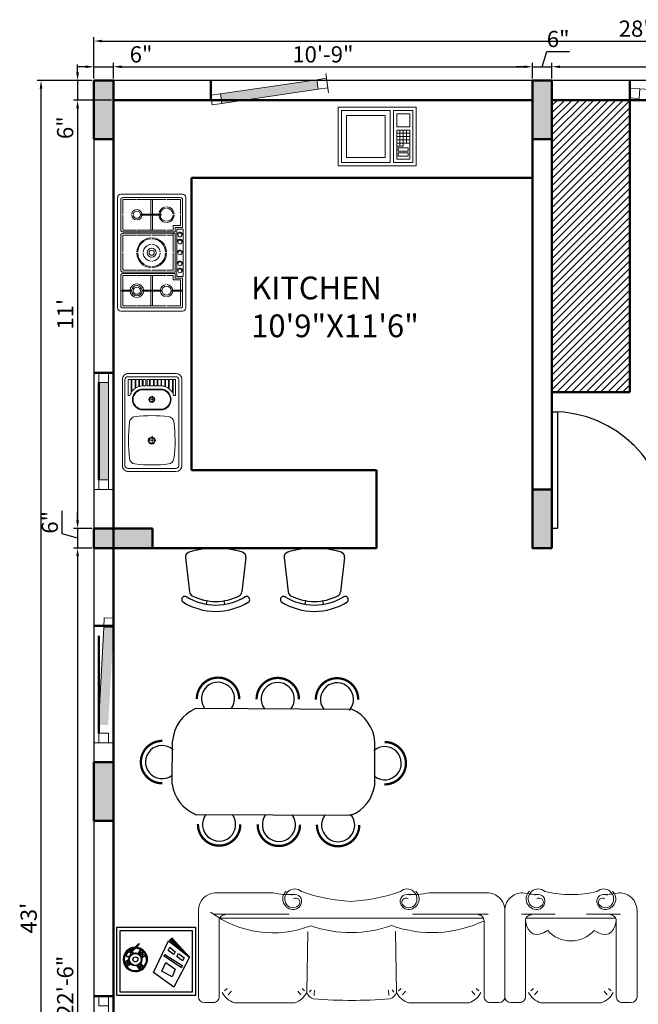
# Model space of a CAD drawing. Units: inches. Extents: x 3064 to 19385, y 846 to 15425.
# Tile 28 of 108: x 4742 to 4932, y 1108 to 1411. Entities that reach past the tile are written whole.
import ezdxf

# ---------------------------------------------------------------- set-up
doc = ezdxf.new("R2010")
doc.units = ezdxf.units.IN
for name, color, linetype, lineweight in [('A-ANNO-DIMS', 2, 'Continuous', 18), ('A-AREA-IDEN', 3, 'Continuous', 18), ('A-COLS', 1, 'Continuous', 35), ('A-DOOR', 3, 'Continuous', 25), ('A-EQPM', 8, 'Continuous', 18), ('A-FLOR-FIXT', 9, 'Continuous', 18), ('A-FURN', 8, 'Continuous', 18), ('A-FURN-PATT', 252, 'Continuous', 13), ('A-GLAZ', 4, 'Continuous', 18), ('A-WALL', 7, 'Continuous', 50), ('C-PROP', 6, 'Continuous', 25)]:
    doc.layers.add(name, color=color, linetype=linetype, lineweight=lineweight)
for name, color, linetype in [('BLO', 135, 'Continuous'), ('FUR', 42, 'Continuous'), ('NOITHAT', 21, 'Continuous'), ('Win', 152, 'Continuous')]:
    doc.layers.add(name, color=color, linetype=linetype)
doc.styles.get("Standard").update_dxf_attribs({"font": 'arial.ttf'})
doc.dimstyles.new('ISO-25', dxfattribs={"dimtxt": 9, "dimasz": 2.5, "dimexe": 1.25, "dimexo": 0.625, "dimtad": 1, "dimdec": 1, "dimlunit": 3, "dimtxsty": 'Standard', "dimcen": 2.5, "dimadec": 0, "dimazin": 0, "dimtfac": 1, "dimtdec": 1, "dimtmove": 0, "dimatfit": 3, "dimfxl": 1, "dimarcsym": 0})

# ---------------------------------------------------------------- blocks, each defined once
blk = doc.blocks.new('*U3')
for p, q in [((0, 0), (0, -6)), ((36, 0), (36, -6))]:
    blk.add_line(p, q)
blk.add_lwpolyline([(0, 0), (0, 36), (1.75, 36), (1.75, 0)], close=True)
blk.add_arc((0, 0), 36, 0, 90)
blk = doc.blocks.new('din')
at = {"layer": 'FUR', "ltscale": 0.25}
for p, q in [((70.23, 15.24), (9.28, 15.24)), ((0, 3.44), (0, -13.56)), ((79.14, 3.44), (79.14, -13.56)), ((8.91, -26.16), (70.23, -26.16))]:
    blk.add_line(p, q, dxfattribs=at)
at = {"layer": 'FUR', "ltscale": 0.25, "const_width": 0.9}
for points in [[(22.5, 19.02, 1.012537), (5.94, 19.02, 1.012537)], [(45.67, 19.02, 1.012537), (29.11, 19.02, 1.012537)], [(69.02, 19.02, 1.012537), (52.46, 19.02, 1.012537)], [(-3.79, 3.1, 1.012537), (-3.79, -13.47, 1.012537)], [(83.08, 3.1, -1.012537), (83.08, -13.47, -1.012537)], [(23.18, -29.95, -1.012537), (6.61, -29.95, -1.012537)], [(46.34, -29.95, -1.012537), (29.78, -29.95, -1.012537)], [(69.7, -29.95, -1.012537), (53.14, -29.95, -1.012537)]]:
    blk.add_lwpolyline(points, format="xyb", dxfattribs=at)
at = {"layer": 'FUR', "ltscale": 0.25}
for centre, radius, start, end in [((14.22, 19.13), 6.48, 323.1301, 221.2163), ((37.39, 19.13), 6.48, 323.1301, 216.8699), ((60.74, 19.13), 6.48, 323.1301, 216.8699), ((14.55, 1.54), 14.67, 111.0491, 172.5731), ((64.59, 1.54), 14.67, 7.4269, 68.9509), ((-3.89, -5.18), 6.48, 53.1301, 311.2163), ((83.18, -5.18), 6.48, 228.7837, 126.8699), ((15.28, -12.21), 15.34, 185.0602, 245.4675), ((63.86, -12.21), 15.34, 294.5325, 354.9398), ((14.89, -30.05), 6.48, 138.7837, 36.8699), ((38.06, -30.05), 6.48, 143.1301, 36.8699), ((61.42, -30.05), 6.48, 143.1301, 36.8699)]:
    blk.add_arc(centre, radius, start, end, dxfattribs=at)
blk = doc.blocks.new('A$C558E769F')
at = {"layer": 'NOITHAT'}
for p, q in [((29.4, 426.4), (61.1, 154.1)), ((508.9, 426.4), (477.2, 154.1)), ((197.1, 55.9), (201.8, 84.2)), ((341.2, 55.9), (336.5, 84.2))]:
    blk.add_line(p, q, dxfattribs=at)
for centre, radius, start, end in [((69.1, 431), 40, 107.02981, 186.63805), ((269.2, -222), 723, 72.97019, 107.02981), ((469.2, 431), 40, 353.36195, 72.97019), ((25.3, 93.7), 25.7, 44.80366, 252.32262), ((269.2, 492.6), 442.6, 237.77056, 302.22944), ((100.8, 158.7), 40, 186.63805, 243.24485), ((269.2, 492.6), 413.9, 243.24485, 296.75515), ((437.5, 158.7), 40, 296.75515, 353.36195), ((513, 93.7), 25.7, 287.67738, 135.19634), ((269.2, 492.6), 492.6, 237.85101, 302.14899)]:
    blk.add_arc(centre, radius, start, end, dxfattribs=at)
blk = doc.blocks.new('sofa-32')
at = {"color": 0, "linetype": 'ByBlock'}
for p, q in [((-0.026, 0.9238), (-0.1, 0.9238)), ((0.657, 0.9252), (0.1531, 0.9252)), ((1.6158, 0.9252), (2.1197, 0.9252)), ((2.3728, 0.9238), (2.2988, 0.9238)), ((-0.15, 0.15), (-0.15, 0.8738)), ((0.024, 0.2361), (0.024, 0.8738)), ((0.05, 0.8375), (0.05, 0.8379)), ((0.1006, 0.8574), (0.1265, 0.8286)), ((0.7096, 0.8574), (0.6837, 0.8286)), ((0.7682, 0.3257), (0.7597, 0.8384)), ((0.7601, 0.8375), (0.7601, 0.8379)), ((0.7823, 0.8346), (0.7966, 0.8162)), ((0.8227, 0.8633), (0.8259, 0.8195)), ((1.4501, 0.8633), (1.447, 0.8195)), ((1.4906, 0.8346), (1.4762, 0.8162)), ((1.5046, 0.3257), (1.5131, 0.8384)), ((1.5127, 0.8375), (1.5127, 0.8379)), ((1.5632, 0.8574), (1.5891, 0.8286)), ((2.1722, 0.8574), (2.1463, 0.8286)), ((2.2228, 0.8375), (2.2228, 0.8379)), ((2.2228, 0.8375), (2.2228, 0.8379)), ((2.2488, 0.2361), (2.2488, 0.8738)), ((2.4228, 0.15), (2.4228, 0.8738)), ((0.0903, 0.8062), (0.0682, 0.8242)), ((0.7199, 0.8062), (0.742, 0.8242)), ((1.5529, 0.8062), (1.5308, 0.8242)), ((2.1825, 0.8062), (2.2046, 0.8242)), ((-0.01, 0.1801), (0.6238, 0.1801)), ((0.0289, 0.2145), (2.2439, 0.2145)), ((2.2948, 0.1801), (1.661, 0.1801)), ((0, 0), (0.4856, 0)), ((2.2848, 0), (1.7991, 0))]:
    blk.add_line(p, q, dxfattribs=at)
at = {"color": 0, "linetype": 'ByBlock', "extrusion": (0, 0, -1)}
for centre, major_axis, start_param, end_param in [((-0.1, 0.8738), (0.0354, 0.0354), 3.926992, 5.497787), ((-0.026, 0.8738), (-0.0354, 0.0354), 0.785398, 2.356196), ((0.1997, 0.7661), (0.1173, 0.1173), 4.372209, 5.213218), ((0.6105, 0.7661), (0.1173, 0.1173), -0.500829, 0.34018), ((1.6624, 0.7661), (0.1173, 0.1173), 4.372209, 5.213218), ((2.0731, 0.7661), (-0.1173, 0.1173), 1.069968, 1.910976), ((2.2988, 0.8738), (-0.0354, 0.0354), 5.497786, 7.068583), ((2.3728, 0.8738), (0.0354, 0.0354), -0.785398, 0.785398), ((0.8378, 0.8143), (-0.0573, 0.0573), 5.78837, 6.779907), ((1.1202, -2.7856), (2.6094, 2.6094), -0.86827, -0.778364), ((1.1526, -2.7856), (2.6094, 2.6094), -0.792432, -0.702526), ((1.435, 0.8143), (-0.0573, 0.0573), 1.074075, 2.065611), ((0.4599, -0.6685), (0.71, 0.71), 5.048761, 5.844539), ((1.1424, -0.6685), (-0.71, 0.71), 0.438646, 1.125824), ((1.7954, -0.5466), (-0.6249, 0.6249), 0.417642, 1.423136), ((0.074, 0.2361), (0.0354, 0.0354), 2.356194, 3.926992), ((2.1988, 0.2361), (0.0354, 0.0354), 0.785397, 2.356194), ((0, 0.15), (0.1061, 0.1061), 2.356194, 3.926992), ((0.6576, 0.0525), (-0.0624, 0.0624), 4.675944, 7.152385), ((0.6708, 0.0524), (-0.059, 0.059), 3.186406, 6.094039), ((0.6552, 0.0629), (0.0458, 0.0458), 4.523242, 6.472337), ((0.6801, 0.0798), (-0.0245, 0.0245), 1.759948, 4.523241), ((0.6592, 0.0712), (-0.0491, 0.0491), 0.8692, 2.230507), ((1.6256, 0.0712), (-0.0491, 0.0491), 5.623477, 6.984784), ((1.614, 0.0524), (0.059, 0.059), 0.189149, 3.096782), ((1.6047, 0.0798), (0.0245, 0.0245), 1.759947, 4.52324), ((1.6295, 0.0629), (0.0458, 0.0458), 4.52324, 6.472335), ((1.6271, 0.0525), (-0.0624, 0.0624), 0.701599, 3.17804), ((2.2728, 0.15), (0.1061, 0.1061), 0.785398, 2.356194), ((0.6324, -0.6613), (-0.479, 0.479), 0.566947, 0.842011), ((0.6701, 0.0726), (0.0414, 0.0414), 0.659711, 2.852687), ((1.2153, -1.3904), (1.0359, 1.0359), 5.158011, 5.447964), ((1.0694, -1.3904), (1.0359, 1.0359), 5.547613, 5.837566), ((1.6147, 0.0726), (-0.0414, 0.0414), 3.430501, 5.623477), ((1.6523, -0.6613), (0.479, 0.479), 5.441177, 5.716241)]:
    blk.add_ellipse(centre, major_axis=major_axis, ratio=1, start_param=start_param, end_param=end_param, dxfattribs=at)
blk = doc.blocks.new('sofa-34')
at = {"color": 0, "linetype": 'ByBlock'}
for p, q in [((-0.026, 0.9238), (-0.1, 0.9238)), ((0.657, 0.9252), (0.1531, 0.9252)), ((0.8361, 0.9238), (0.9101, 0.9238)), ((-0.15, 0.15), (-0.15, 0.8738)), ((0.024, 0.2361), (0.024, 0.8738)), ((0.05, 0.8375), (0.05, 0.8379)), ((0.1006, 0.8574), (0.1265, 0.8286)), ((0.7096, 0.8574), (0.6837, 0.8286)), ((0.7601, 0.8375), (0.7601, 0.8379)), ((0.7602, 0.8375), (0.7601, 0.8379)), ((0.7861, 0.2361), (0.7861, 0.8738)), ((0.9601, 0.15), (0.9601, 0.8738)), ((0.0903, 0.8062), (0.0682, 0.8242)), ((0.7199, 0.8062), (0.742, 0.8242)), ((-0.01, 0.1801), (0.2738, 0.1801)), ((0.0289, 0.2145), (0.7812, 0.2145)), ((0.8201, 0.1801), (0.5364, 0.1801))]:
    blk.add_line(p, q, dxfattribs=at)
blk.add_arc((0.4051, 0.1479), 0.2579, 40.79835, 139.20165, dxfattribs=at)
at = {"color": 0, "linetype": 'ByBlock', "extrusion": (0, 0, -1)}
for centre, major_axis, ratio, start_param, end_param in [((-0.1, 0.8738), (0.0354, 0.0354), 1, 3.926992, 5.497787), ((-0.026, 0.8738), (-0.0354, 0.0354), 1, 0.785398, 2.356196), ((0.1997, 0.7661), (0.1173, 0.1173), 1, 4.372209, 5.213218), ((0.6105, 0.7661), (0.1173, 0.1173), 1, -0.500829, 0.34018), ((0.5004, -0.5869), (-0.4145, 0.931), 0.264583, -0.381915, 0.387685), ((0.074, 0.2361), (-0.0354, 0.0354), 1, 3.926991, 5.497788), ((0, 0.15), (0.1061, 0.1061), 1, 2.356194, 3.926992), ((0.1167, 0.0525), (-0.0624, 0.0624), 1, 4.675944, 7.152385), ((0.1299, 0.0524), (-0.059, 0.059), 1, 3.186406, 6.094039), ((0.1144, 0.0629), (-0.0458, 0.0458), 1, 6.094039, 8.043134), ((0.1392, 0.0798), (0.0245, 0.0245), 1, 0.189152, 2.952444), ((0.1183, 0.0712), (0.0491, 0.0491), 1, -0.701597, 0.659711), ((0.179, -0.6576), (-0.2506, 0.635), 0.885019, 0.124301, 0.339591), ((0.1292, 0.0726), (-0.0414, 0.0414), 1, 2.230507, 4.423483), ((0.3517, -0.5578), (0.7346, 0.1067), 0.76838, 4.597815, 5.20076)]:
    blk.add_ellipse(centre, major_axis=major_axis, ratio=ratio, start_param=start_param, end_param=end_param, dxfattribs=at)
at = {"color": 0, "linetype": 'ByBlock'}
for centre, major_axis, ratio, start_param, end_param in [((0.8361, 0.8738), (0.0354, 0.0354), 1, 0.785398, 2.356196), ((0.9101, 0.8738), (-0.0354, 0.0354), 1, 3.926992, 5.497787), ((0.3097, -0.5869), (0.4145, 0.931), 0.264583, -0.381915, 0.387685), ((0.7361, 0.2361), (0.0354, 0.0354), 1, 3.926991, 5.497788), ((0.6918, 0.0712), (-0.0491, 0.0491), 1, -0.701597, 0.659711), ((0.6802, 0.0524), (0.059, 0.059), 1, 3.186406, 6.094039), ((0.6709, 0.0798), (-0.0245, 0.0245), 1, 0.189152, 2.952444), ((0.6958, 0.0629), (0.0458, 0.0458), 1, 6.094039, 8.043134), ((0.6934, 0.0525), (0.0624, 0.0624), 1, 4.675944, 7.152385), ((0.8101, 0.15), (-0.1061, 0.1061), 1, 2.356194, 3.926992), ((0.6809, 0.0726), (0.0414, 0.0414), 1, 2.230507, 4.423483), ((0.6312, -0.6576), (0.2506, 0.635), 0.885019, 0.124301, 0.339591)]:
    blk.add_ellipse(centre, major_axis=major_axis, ratio=ratio, start_param=start_param, end_param=end_param, dxfattribs=at)
blk = doc.blocks.new('sink 1')
for points in [[(-7.34, 1.48), (-7.34, 22.73)], [(-6.56, 1.48), (-6.56, 22.73)], [(5.86, 24.22), (-5.86, 24.22)], [(6.01, 23.43), (-5.86, 23.43)], [(6.72, 1.48), (6.72, 22.73)], [(7.34, 1.48), (7.34, 22.73)], [(0, 15.39), (0, 17.42)], [(1.09, 16.48), (-0.94, 16.48)], [(-2.09, 8.99), (2.28, 8.99)], [(-2.09, 8.84), (2.28, 8.84)], [(-5.78, 5.39), (-5.78, 5.39)], [(-5.31, 5.39), (-5.31, 5.39)], [(-5.16, 4.92), (-5.16, 4.92)], [(0.78, 6.33), (-0.78, 6.33)], [(0, 5.55), (0, 7.26)], [(5.16, 4.92), (5.16, 4.92)], [(5.94, 5.39), (5.94, 5.39)], [(-5, 1.48), (-5, 4.69)], [(-5, 1.48), (-4.22, 1.48), (-4.22, 3.83)], [(-4.84, 4.45), (-4.84, 4.45)], [(-4.22, 3.83), (-4.22, 3.83)], [(-4.06, 1.48), (-4.06, 3.69)], [(-4.06, 1.48), (-3.28, 1.48), (-3.28, 3.27)], [(-3.91, 3.52), (-3.91, 3.52)], [(-3.28, 3.2), (-3.28, 3.2)], [(-3.12, 3.2), (-3.12, 3.2)], [(-2.34, 3.05), (-2.34, 3.05)], [(-2.19, 3.05), (-2.19, 3.05)], [(-2.09, 3.99), (2.28, 3.99)], [(-2.09, 3.84), (2.28, 3.84)], [(-1.41, 3.05), (-1.41, 3.05)], [(-1.25, 3.05), (-1.25, 3.05)], [(-0.47, 1.48), (-1.25, 1.48), (-1.25, 3.05), (-0.47, 3.05)], [(-0.62, 3.05), (-0.62, 3.05)], [(-0.47, 1.48), (-0.47, 3.05)], [(-0.31, 3.05), (-0.31, 3.05)], [(0.47, 1.48), (-0.31, 1.48), (-0.31, 3.05), (0.47, 3.05)], [(0.31, 3.05), (0.31, 3.05)], [(0.47, 1.48), (0.47, 3.05)], [(0.62, 3.05), (0.62, 3.05)], [(1.25, 3.05), (1.25, 3.05)], [(1.56, 3.05), (1.56, 3.05)], [(2.19, 3.05), (2.19, 3.05)], [(2.5, 3.05), (2.5, 3.05)], [(3.12, 3.2), (3.12, 3.2)], [(3.28, 1.48), (4.06, 1.48), (4.06, 3.57)], [(3.28, 1.48), (3.28, 3.2)], [(3.44, 3.2), (3.44, 3.2)], [(4.06, 3.52), (4.06, 3.52)], [(4.22, 1.48), (4.22, 3.67)], [(4.37, 3.83), (4.37, 3.83)], [(5, 4.45), (5, 4.45)], [(6.01, 0.78), (-5.86, 0.78)], [(5.86, 0), (-5.86, 0)], [(-5.78, 1.48), (-5.78, 1.48)], [(-5.16, 1.48), (-5.16, 1.48)], [(-4.84, 1.48), (-4.84, 1.48)], [(-4.22, 1.48), (-4.22, 1.48)], [(-3.91, 1.48), (-3.91, 1.48)], [(-3.28, 1.48), (-3.28, 1.48)], [(-3.12, 1.48), (-3.12, 1.48)], [(-2.34, 1.48), (-2.34, 1.48)], [(-2.19, 1.48), (-2.19, 1.48)], [(-1.41, 1.48), (-1.41, 1.48)], [(-1.25, 1.48), (-1.25, 1.48)], [(-0.62, 1.48), (-0.62, 1.48)], [(-0.31, 1.48), (-0.31, 1.48)], [(0.31, 1.48), (0.31, 1.48)], [(0.62, 1.48), (0.62, 1.48)], [(1.25, 1.48), (1.25, 1.48)], [(1.56, 1.48), (1.56, 1.48)], [(2.19, 1.48), (2.19, 1.48)], [(2.5, 1.48), (2.5, 1.48)], [(3.12, 1.48), (3.12, 1.48)], [(3.44, 1.48), (3.44, 1.48)], [(4.06, 1.48), (4.06, 1.48)], [(4.37, 1.48), (4.37, 1.48)], [(5, 1.48), (5, 1.48)], [(5.16, 1.48), (5.16, 1.48)], [(5.94, 1.48), (5.94, 1.48)]]:
    blk.add_lwpolyline(points)
for points in [[(-5.16, 4.92), (-5.16, 1.48), (-5.78, 1.48), (-5.78, 5.39), (-5.31, 5.39, -0.068511), (-5.16, 4.92)], [(5.16, 4.92, 0.248301), (5.47, 5.39), (5.94, 5.39), (5.94, 1.48), (5.16, 1.48), (5.16, 4.92)], [(4.06, 3.57, -0.061679), (3.32, 3.22)], [(4.22, 1.48), (5, 1.48), (5, 4.45, -0.083542), (4.22, 3.67, -0.083542)]]:
    blk.add_lwpolyline(points, format="xyb")
for points in [[(-3.12, 3.22), (-3.12, 1.48), (-2.34, 1.48), (-2.34, 3.05, -0.06228)], [(2.5, 3.05), (2.5, 1.48), (3.12, 1.48), (3.12, 3.2, -0.050256)]]:
    blk.add_lwpolyline(points, format="xyb", close=True)
for points in [[(-2.19, 3.05), (-1.41, 3.05), (-1.41, 1.48), (-2.19, 1.48)], [(0.62, 3.05), (1.25, 3.05), (1.25, 1.48), (0.62, 1.48)], [(2.19, 1.48), (2.19, 3.05), (1.56, 3.05), (1.56, 1.48)]]:
    blk.add_lwpolyline(points, close=True)
for centre, radius in [((0.09, 16.57), 0.859), ((0.09, 16.57), 0.703), ((0.09, 6.41), 0.703), ((0.09, 6.41), 0.547)]:
    blk.add_circle(centre, radius)
for centre, radius, start, end in [((-5.86, 22.73), 1.48, 90, 180), ((-5.86, 22.73), 0.703, 90, 180), ((-3.87, 20.82), 1.53, 97.3256, 171.1849), ((0.09, -12.65), 35.23, 83.2159, 96.7841), ((4.06, 20.82), 1.53, 8.8151, 82.6744), ((5.86, 22.73), 1.48, 360, 90), ((6.01, 22.73), 0.703, 0, 90), ((30.19, 16.56), 35.85, 172.7947, 187.4213), ((-30, 16.56), 35.85, 352.5787, 7.2053), ((-3.89, 12.12), 1.48, 187.4212, 263.2159), ((0.09, 45.63), 35.23, 263.2159, 276.7841), ((4.08, 12.12), 1.48, 276.7841, 352.5788), ((-2.1, 6.41), 2.58, 90, 270), ((-2.1, 6.41), 2.42, 90, 270), ((2.28, 6.41), 2.58, 270, 90), ((2.28, 6.41), 2.42, 270, 90), ((-2.15, 6.48), 3.36, 212.1095, 232.0862), ((-2.1, 6.41), 3.36, 234.156, 249.3275), ((2.14, 6.36), 3.36, 289.8633, 290.5971), ((-5.86, 1.48), 1.48, 180, 270), ((-5.86, 1.48), 0.703, 180, 270), ((5.86, 1.48), 1.48, 270, 0), ((6.01, 1.48), 0.703, 270, 360)]:
    blk.add_arc(centre, radius, start, end)
blk = doc.blocks.new('STOVE')
for p, q in [((11.85, 19.7), (11.55, 19.7)), ((11.55, 16.92), (11.55, 19.7)), ((11.85, 16.92), (11.85, 19.7)), ((11.85, 16.92), (11.55, 16.92)), ((-11.85, 13.73), (-11.85, 7.62)), ((-11.85, 13.73), (-11.55, 13.73)), ((-11.55, 13.73), (-11.55, 7.62)), ((11.85, 13.23), (11.55, 13.23)), ((11.55, 13.23), (11.55, 7.57)), ((11.85, 13.23), (11.85, 7.57)), ((-11.85, 10.75), (-16.4, 10.75)), ((-11.85, 10.25), (-16.4, 10.25)), ((-7, 10.75), (-11.55, 10.75)), ((-7, 10.25), (-11.55, 10.25)), ((7, 10.75), (11.55, 10.75)), ((7, 10.25), (11.55, 10.25)), ((11.85, 10.75), (16.4, 10.75)), ((11.85, 10.25), (16.4, 10.25)), ((-11.85, 7.62), (-11.55, 7.62)), ((11.85, 7.57), (11.55, 7.57)), ((-7, 3.9), (-8.4, 3.9)), ((-7.8, 3.3), (-7.8, 1)), ((-6.4, 3.3), (-7.8, 3.3)), ((-5.4, 3.9), (-6, 3.9)), ((-5.4, 3.9), (-0.15, 3.9)), ((0.15, 3.9), (5.4, 3.9)), ((6.4, 3.3), (7.8, 3.3)), ((7, 3.9), (8.4, 3.9)), ((7.8, 3.3), (7.8, 1)), ((8.4, 3.9), (8.4, 1.6)), ((11.85, 4.28), (11.55, 4.28)), ((11.55, 4.28), (11.55, 1.3)), ((11.85, 4.28), (11.85, 1.3)), ((7.3, 2.8), (-7.3, 2.8)), ((-7.3, 2.8), (-7.3, 0.8)), ((7.3, 0.8), (-7.3, 0.8)), ((7.3, 2.8), (7.3, 0.8)), ((11.85, 1.3), (11.55, 1.3))]:
    blk.add_line(p, q)
for points in [[(-17, 21), (17, 21, -0.414214), (18, 20), (18, 1, -0.414214), (17, 0), (-17, 0, -0.414214), (-18, 1), (-18, 20, -0.414214)], [(6, 3.3), (-6, 3.3), (-6, 19.4, -0.414214), (-5.4, 20), (5.4, 20, -0.414214), (6, 19.4)]]:
    blk.add_lwpolyline(points, format="xyb", close=True)
for points in [[(-7.8, 1), (-16.4, 1, -0.414214), (-17, 1.6), (-17, 19.4, -0.414214), (-16.4, 20), (-7, 20, -0.414214), (-6.4, 19.4), (-6.4, 3.3)], [(6.4, 19.4, -0.414214), (7, 20), (16.4, 20, -0.414214), (17, 19.4), (17, 1.6, -0.414214), (16.4, 1), (7.8, 1)]]:
    blk.add_lwpolyline(points, format="xyb")
for points in [[(-16.4, 15.22), (-16.4, 19.4), (-11.85, 19.4)], [(-11.55, 19.4), (-7, 19.4), (-7, 15.22)], [(-5.4, 15.22), (-5.4, 19.4), (-0.15, 19.4)], [(0.15, 19.4), (5.4, 19.4), (5.4, 15.22)], [(6.4, 3.3), (6.4, 19.4)], [(7, 15.22), (7, 19.4), (11.55, 19.4)], [(11.85, 19.4), (16.4, 19.4), (16.4, 15.22)], [(-16.4, 6.08), (-16.4, 14.92)], [(-7, 14.92), (-7, 6.08)], [(-5.4, 10.65), (-5.4, 14.92)], [(5.4, 14.92), (5.4, 10.65)], [(7, 6.08), (7, 14.92)], [(16.4, 14.92), (16.4, 6.08)], [(-5.4, 6.08), (-5.4, 10.35)], [(5.4, 10.35), (5.4, 6.08)], [(-11.85, 1.6), (-16.4, 1.6), (-16.4, 5.77)], [(-8.4, 3.9), (-8.4, 1.6), (-11.55, 1.6)], [(-7, 5.77), (-7, 3.9)], [(-5.4, 3.9), (-5.4, 5.77)], [(5.4, 5.77), (5.4, 3.9)], [(7, 3.9), (7, 5.77)], [(16.4, 5.77), (16.4, 1.6), (11.85, 1.6)], [(11.55, 1.6), (8.4, 1.6)]]:
    blk.add_lwpolyline(points)
for centre, radius in [((-11.7, 15.07), 1.1), ((11.7, 15.07), 1.6), ((11.7, 15.07), 1.1), ((0, 10.5), 1.4), ((0, 10.5), 0.8), ((11.7, 5.93), 1.4), ((-5.49, 1.8), 0.6), ((-3.3, 1.8), 0.6), ((0, 1.8), 0.6), ((3.39, 1.8), 0.6), ((5.57, 1.8), 0.6)]:
    blk.add_circle(centre, radius)
for centre, radius, start, end in [((-11.7, 15.07), 1.6, 95.3794, 174.6206), ((-11.7, 15.07), 1.6, 5.3794, 84.6206), ((11.7, 15.07), 2.1, 94.096, 175.904), ((11.7, 15.07), 2.1, 4.096, 85.904), ((-11.7, 15.07), 1.6, 185.3794, 264.6206), ((-11.7, 15.07), 1.6, 275.3794, 354.6206), ((0, 10.5), 4.6, 91.8687, 178.1313), ((0, 10.5), 4.3, 91.9991, 178.0009), ((0, 10.5), 2.6, 93.3074, 176.6926), ((0, 10.5), 4.6, 1.8687, 88.1313), ((0, 10.5), 4.3, 1.9991, 88.0009), ((0, 10.5), 2.6, 3.3074, 86.6926), ((11.7, 15.07), 2.1, 184.096, 265.904), ((11.7, 15.07), 2.1, 274.096, 355.904), ((0, 10.5), 4.6, 181.8687, 268.1313), ((0, 10.5), 4.3, 181.9991, 268.0009), ((0, 10.5), 2.6, 183.3074, 266.6926), ((0, 10.5), 4.6, 271.8687, 358.1313), ((0, 10.5), 4.3, 271.9991, 358.0009), ((0, 10.5), 2.6, 273.3074, 356.6926), ((-11.7, 5.93), 2.4, 93.5833, 176.4167), ((-11.7, 5.93), 2, 94.3012, 175.6988), ((-11.7, 5.93), 2.4, 3.5833, 86.4167), ((-11.7, 5.93), 2, 4.3012, 85.6988), ((11.7, 5.93), 1.9, 94.5281, 175.4719), ((11.7, 5.93), 1.9, 4.5281, 85.4719), ((-11.7, 5.93), 2.4, 183.5833, 266.4167), ((-11.7, 5.93), 2, 184.3012, 265.6988), ((-11.7, 5.93), 2.4, 273.5833, 356.4167), ((-11.7, 5.93), 2, 274.3012, 355.6988), ((11.7, 5.93), 1.9, 184.5281, 265.4719), ((11.7, 5.93), 1.9, 274.5281, 355.4719), ((-5.49, 1.8), 0.846, 89.9979, 270), ((-3.3, 1.8), 0.846, 89.9979, 270), ((0, 1.8), 0.846, 89.9979, 270), ((3.39, 1.8), 0.846, 89.9979, 270), ((5.57, 1.8), 0.846, 89.9979, 270)]:
    blk.add_arc(centre, radius, start, end)
blk = doc.blocks.new('Microwave')
for p, q in [((18, 10), (22, 10)), ((19, 7), (19, 11)), ((20, 11), (20, 7)), ((21, 7), (21, 11)), ((22, 9), (18, 9)), ((18, 8), (22, 8)), ((22, 7), (18, 7)), ((19, 6), (19, 7)), ((20, 7), (20, 6)), ((20, 6), (18, 6))]:
    blk.add_line(p, q)
for points in [[(0, 0), (0, 18), (24, 18), (24, 0)], [(1, 1), (1, 17), (16, 17), (16, 1)], [(2.5, 2.5), (2.5, 15.5), (14.5, 15.5), (14.5, 2.5)], [(17, 1), (17, 17), (23, 17), (23, 1)], [(18, 12), (18, 16), (22, 16), (22, 12)], [(18, 2), (18, 11), (22, 11), (22, 2)], [(18.5, 4.5), (18.5, 5.5), (21.5, 5.5), (21.5, 4.5)], [(18.5, 3), (18.5, 4), (21.5, 4), (21.5, 3)]]:
    blk.add_lwpolyline(points, close=True)
blk = doc.blocks.new('*D43')
at = {"layer": 'A-ANNO-DIMS', "color": 0, "lineweight": -2, "transparency": 16777216}
for p, q in [((4761.98, 1396.35), (4759.48, 1396.35)), ((4764.48, 1392.72), (4764.48, 1397.6)), ((4764.48, 1396.35), (4770.48, 1396.35)), ((4770.48, 1392.72), (4770.48, 1397.6)), ((4772.98, 1396.35), (4782.5, 1396.35))]:
    blk.add_line(p, q, dxfattribs=at)
at = {"layer": 'A-ANNO-DIMS', "color": 0, "transparency": 16777216}
for points in [[(4761.98, 1396.77), (4761.98, 1395.93), (4764.48, 1396.35)], [(4772.98, 1396.77), (4772.98, 1395.93), (4770.48, 1396.35)]]:
    blk.add_solid(points, dxfattribs=at)
at = {"layer": 'Defpoints', "color": 0, "transparency": 16777216}
for p in [(4770.48, 1396.35), (4764.48, 1392.1), (4770.48, 1392.1)]:
    blk.add_point(p, dxfattribs=at)
at = {"layer": 'A-ANNO-DIMS', "color": 0, "transparency": 16777216, "insert": (4778.99, 1399.53), "char_height": 5, "attachment_point": 5}
blk.add_mtext('6"', dxfattribs=at)
blk = doc.blocks.new('*D44')
at = {"layer": 'A-ANNO-DIMS', "color": 0, "lineweight": -2, "transparency": 16777216}
for p, q in [((4770.48, 1392.72), (4770.48, 1397.6)), ((4772.98, 1396.35), (4896.98, 1396.35)), ((4899.48, 1392.72), (4899.48, 1397.6))]:
    blk.add_line(p, q, dxfattribs=at)
at = {"layer": 'A-ANNO-DIMS', "color": 0, "transparency": 16777216}
for points in [[(4772.98, 1396.77), (4772.98, 1395.93), (4770.48, 1396.35)], [(4896.98, 1396.77), (4896.98, 1395.93), (4899.48, 1396.35)]]:
    blk.add_solid(points, dxfattribs=at)
at = {"layer": 'Defpoints', "color": 0, "transparency": 16777216}
for p in [(4899.48, 1396.35), (4770.48, 1392.1), (4899.48, 1392.1)]:
    blk.add_point(p, dxfattribs=at)
at = {"layer": 'A-ANNO-DIMS', "color": 0, "transparency": 16777216, "insert": (4834.98, 1399.53), "char_height": 5, "attachment_point": 5}
blk.add_mtext('10\'-9"', dxfattribs=at)
blk = doc.blocks.new('*D45')
at = {"layer": 'A-ANNO-DIMS', "color": 0, "lineweight": -2, "transparency": 16777216}
for p, q in [((4902.48, 1396.35), (4903.9, 1401.09)), ((4903.9, 1401.09), (4910.92, 1401.09)), ((4896.98, 1396.35), (4894.48, 1396.35)), ((4899.48, 1392.72), (4899.48, 1397.6)), ((4899.48, 1396.35), (4905.48, 1396.35)), ((4899.48, 1396.35), (4905.48, 1396.35)), ((4905.48, 1392.72), (4905.48, 1397.6)), ((4907.98, 1396.35), (4910.48, 1396.35))]:
    blk.add_line(p, q, dxfattribs=at)
at = {"layer": 'A-ANNO-DIMS', "color": 0, "transparency": 16777216}
for points in [[(4896.98, 1396.77), (4896.98, 1395.93), (4899.48, 1396.35)], [(4907.98, 1396.77), (4907.98, 1395.93), (4905.48, 1396.35)]]:
    blk.add_solid(points, dxfattribs=at)
at = {"layer": 'Defpoints', "color": 0, "transparency": 16777216}
for p in [(4905.48, 1396.35), (4899.48, 1392.1), (4905.48, 1392.1)]:
    blk.add_point(p, dxfattribs=at)
at = {"layer": 'A-ANNO-DIMS', "color": 0, "transparency": 16777216, "insert": (4907.41, 1404.27), "char_height": 5, "attachment_point": 5}
blk.add_mtext('6"', dxfattribs=at)
blk = doc.blocks.new('*D46')
at = {"layer": 'A-ANNO-DIMS', "color": 0, "lineweight": -2, "transparency": 16777216}
for p, q in [((4905.48, 1392.72), (4905.48, 1397.6)), ((4907.98, 1396.35), (5097.98, 1396.35)), ((5100.48, 1392.72), (5100.48, 1397.6))]:
    blk.add_line(p, q, dxfattribs=at)
at = {"layer": 'A-ANNO-DIMS', "color": 0, "transparency": 16777216}
for points in [[(4907.98, 1396.77), (4907.98, 1395.93), (4905.48, 1396.35)], [(5097.98, 1396.77), (5097.98, 1395.93), (5100.48, 1396.35)]]:
    blk.add_solid(points, dxfattribs=at)
at = {"layer": 'Defpoints', "color": 0, "transparency": 16777216}
for p in [(5100.48, 1396.35), (4905.48, 1392.1), (5100.48, 1392.1)]:
    blk.add_point(p, dxfattribs=at)
at = {"layer": 'A-ANNO-DIMS', "color": 0, "transparency": 16777216, "insert": (5002.98, 1399.53), "char_height": 5, "attachment_point": 5}
blk.add_mtext('16\'-3"', dxfattribs=at)
blk = doc.blocks.new('*D48')
at = {"layer": 'A-ANNO-DIMS', "color": 0, "lineweight": -2, "transparency": 16777216}
for p, q in [((4759.45, 1394.6), (4759.45, 1397.1)), ((4763.85, 1392.1), (4758.2, 1392.1)), ((4759.45, 1392.1), (4759.45, 1386.1)), ((4769.85, 1386.1), (4758.2, 1386.1)), ((4759.45, 1383.6), (4759.45, 1374.07))]:
    blk.add_line(p, q, dxfattribs=at)
at = {"layer": 'A-ANNO-DIMS', "color": 0, "transparency": 16777216}
for points in [[(4759.03, 1394.6), (4759.86, 1394.6), (4759.45, 1392.1)], [(4759.03, 1383.6), (4759.86, 1383.6), (4759.45, 1386.1)]]:
    blk.add_solid(points, dxfattribs=at)
at = {"layer": 'Defpoints', "color": 0, "transparency": 16777216}
for p in [(4764.48, 1392.1), (4759.45, 1386.1), (4770.48, 1386.1)]:
    blk.add_point(p, dxfattribs=at)
at = {"layer": 'A-ANNO-DIMS', "color": 0, "transparency": 16777216, "insert": (4756.27, 1377.58), "char_height": 5, "attachment_point": 5, "rotation": 90}
blk.add_mtext('6"', dxfattribs=at)
blk = doc.blocks.new('*D49')
at = {"layer": 'A-ANNO-DIMS', "color": 0, "lineweight": -2, "transparency": 16777216}
for p, q in [((4769.85, 1386.1), (4758.2, 1386.1)), ((4759.45, 1383.6), (4759.45, 1256.6)), ((4763.85, 1254.1), (4758.2, 1254.1))]:
    blk.add_line(p, q, dxfattribs=at)
at = {"layer": 'A-ANNO-DIMS', "color": 0, "transparency": 16777216}
for points in [[(4759.03, 1383.6), (4759.86, 1383.6), (4759.45, 1386.1)], [(4759.03, 1256.6), (4759.86, 1256.6), (4759.45, 1254.1)]]:
    blk.add_solid(points, dxfattribs=at)
at = {"layer": 'Defpoints', "color": 0, "transparency": 16777216}
for p in [(4770.48, 1386.1), (4759.45, 1254.1), (4764.48, 1254.1)]:
    blk.add_point(p, dxfattribs=at)
at = {"layer": 'A-ANNO-DIMS', "color": 0, "transparency": 16777216, "insert": (4756.31, 1320.1), "char_height": 5, "attachment_point": 5, "rotation": 90}
blk.add_mtext("11'", dxfattribs=at)
blk = doc.blocks.new('*D50')
at = {"layer": 'A-ANNO-DIMS', "color": 0, "lineweight": -2, "transparency": 16777216}
for p, q in [((4754.71, 1252.52), (4754.71, 1259.54)), ((4759.45, 1256.6), (4759.45, 1259.1)), ((4763.85, 1254.1), (4758.2, 1254.1)), ((4759.45, 1254.1), (4759.45, 1248.1)), ((4759.45, 1254.1), (4759.45, 1248.1)), ((4759.45, 1251.1), (4754.71, 1252.52)), ((4763.85, 1248.1), (4758.2, 1248.1)), ((4759.45, 1245.6), (4759.45, 1243.1))]:
    blk.add_line(p, q, dxfattribs=at)
at = {"layer": 'A-ANNO-DIMS', "color": 0, "transparency": 16777216}
for points in [[(4759.03, 1256.6), (4759.86, 1256.6), (4759.45, 1254.1)], [(4759.03, 1245.6), (4759.86, 1245.6), (4759.45, 1248.1)]]:
    blk.add_solid(points, dxfattribs=at)
at = {"layer": 'Defpoints', "color": 0, "transparency": 16777216}
for p in [(4764.48, 1254.1), (4759.45, 1248.1), (4764.48, 1248.1)]:
    blk.add_point(p, dxfattribs=at)
at = {"layer": 'A-ANNO-DIMS', "color": 0, "transparency": 16777216, "insert": (4751.53, 1256.03), "char_height": 5, "attachment_point": 5, "rotation": 90}
blk.add_mtext('6"', dxfattribs=at)
blk = doc.blocks.new('*D51')
at = {"layer": 'A-ANNO-DIMS', "color": 0, "lineweight": -2, "transparency": 16777216}
for p, q in [((4763.85, 1248.1), (4758.2, 1248.1)), ((4759.45, 1245.6), (4759.45, 980.6)), ((4769.85, 978.1), (4758.2, 978.1))]:
    blk.add_line(p, q, dxfattribs=at)
at = {"layer": 'A-ANNO-DIMS', "color": 0, "transparency": 16777216}
for points in [[(4759.03, 1245.6), (4759.86, 1245.6), (4759.45, 1248.1)], [(4759.03, 980.6), (4759.86, 980.6), (4759.45, 978.1)]]:
    blk.add_solid(points, dxfattribs=at)
at = {"layer": 'Defpoints', "color": 0, "transparency": 16777216}
for p in [(4764.48, 1248.1), (4759.45, 978.1), (4770.48, 978.1)]:
    blk.add_point(p, dxfattribs=at)
at = {"layer": 'A-ANNO-DIMS', "color": 0, "transparency": 16777216, "insert": (4756.27, 1113.1), "char_height": 5, "attachment_point": 5, "rotation": 90}
blk.add_mtext('22\'-6"', dxfattribs=at)
blk = doc.blocks.new('*D55')
at = {"layer": 'A-ANNO-DIMS', "color": 0, "lineweight": -2, "transparency": 16777216}
for p, q in [((4763.85, 1392.1), (4746.96, 1392.1)), ((4748.21, 878.6), (4748.21, 1389.6)), ((4763.85, 876.1), (4746.96, 876.1))]:
    blk.add_line(p, q, dxfattribs=at)
at = {"layer": 'A-ANNO-DIMS', "color": 0, "transparency": 16777216}
for points in [[(4747.79, 1389.6), (4748.63, 1389.6), (4748.21, 1392.1)], [(4747.79, 878.6), (4748.63, 878.6), (4748.21, 876.1)]]:
    blk.add_solid(points, dxfattribs=at)
at = {"layer": 'Defpoints', "color": 0, "transparency": 16777216}
for p in [(4748.21, 1392.1), (4764.48, 1392.1), (4764.48, 876.1)]:
    blk.add_point(p, dxfattribs=at)
at = {"layer": 'A-ANNO-DIMS', "color": 0, "transparency": 16777216, "insert": (4745.03, 1134.1), "char_height": 5, "attachment_point": 5, "rotation": 90}
blk.add_mtext("43'", dxfattribs=at)
blk = doc.blocks.new('*D67')
at = {"layer": 'A-ANNO-DIMS', "color": 0, "lineweight": -2, "transparency": 16777216}
for p, q in [((4764.48, 1392.72), (4764.48, 1405.52)), ((5106.48, 1392.72), (5106.48, 1405.52)), ((4766.98, 1404.27), (5103.98, 1404.27))]:
    blk.add_line(p, q, dxfattribs=at)
at = {"layer": 'A-ANNO-DIMS', "color": 0, "transparency": 16777216}
for points in [[(4766.98, 1404.69), (4766.98, 1403.85), (4764.48, 1404.27)], [(5103.98, 1404.69), (5103.98, 1403.85), (5106.48, 1404.27)]]:
    blk.add_solid(points, dxfattribs=at)
at = {"layer": 'Defpoints', "color": 0, "transparency": 16777216}
for p in [(5106.48, 1404.27), (4764.48, 1392.1), (5106.48, 1392.1)]:
    blk.add_point(p, dxfattribs=at)
at = {"layer": 'A-ANNO-DIMS', "color": 0, "transparency": 16777216, "insert": (4935.48, 1407.45), "char_height": 5, "attachment_point": 5}
blk.add_mtext('28\'-6"', dxfattribs=at)
blk = doc.blocks.new('ST1')
at = {"layer": 'BLO'}
for p, q in [((2.87, 1.65), (2.87, 24.72)), ((2.87, 24.72), (22.87, 24.72)), ((3.87, 2.65), (3.87, 23.72)), ((3.87, 23.72), (21.87, 23.72)), ((21.87, 23.72), (21.87, 2.65)), ((22.87, 24.72), (22.87, 1.65)), ((22.87, 1.65), (2.87, 1.65)), ((21.87, 2.65), (3.87, 2.65))]:
    blk.add_line(p, q, dxfattribs=at)
at = {"layer": 'Win'}
for p, q in [((11.4, 21.86), (12.09, 20.65)), ((11.51, 21.94), (12.19, 20.74)), ((11.57, 21.85), (13.19, 21.3)), ((12.55, 22.44), (12.13, 20.85)), ((12.55, 22.44), (13.25, 21.19)), ((12.69, 22.48), (13.4, 21.2)), ((14.51, 20.87), (14.54, 20.9)), ((14.64, 20.77), (14.67, 20.79)), ((15.43, 20.61), (15.22, 19.97)), ((15.22, 19.97), (15.71, 20.33)), ((15.27, 19.81), (15.82, 20.21)), ((15.37, 21.5), (15.64, 21.7)), ((15.41, 20.64), (17.8, 18.17)), ((15.46, 21.36), (15.76, 21.58)), ((15.54, 20.8), (16.34, 20.79)), ((15.54, 20.77), (18.02, 18.4)), ((15.76, 21.58), (15.55, 20.96)), ((17.88, 18.31), (15.58, 20.6)), ((15.87, 20.45), (16.34, 20.79)), ((15.99, 20.33), (16.41, 20.64)), ((10.46, 17.93), (11.6, 18.76)), ((10.53, 17.78), (11.65, 18.59)), ((10.53, 17.78), (12.23, 17.8)), ((11.59, 18.54), (11.11, 16.99)), ((11.11, 16.99), (12.23, 17.8)), ((11.23, 16.87), (12.37, 17.7)), ((13.9, 17.44), (14.58, 16.23)), ((14.03, 17.48), (14.71, 16.28)), ((14.09, 17.38), (15.67, 16.91)), ((15.04, 18.04), (14.71, 16.28)), ((14.97, 18.16), (15.67, 16.91)), ((15, 18.22), (15.87, 17.69)), ((15.13, 18.43), (16.01, 17.9)), ((15.14, 18.13), (15.77, 17.01)), ((5.28, 8.07), (9.58, 13.93)), ((8.3, 8.54), (10.02, 11.57)), ((9.58, 13.93), (18.91, 9.59)), ((10.02, 11.57), (12.5, 10.4)), ((12.5, 10.4), (10.58, 7.59)), ((10.98, 5.74), (14.34, 10.89)), ((14.87, 10.68), (11.67, 5.58)), ((18.91, 9.59), (14.09, 3.45)), ((14.09, 3.45), (19.17, 9.31)), ((14.09, 3.45), (19.44, 9.01)), ((14.09, 3.45), (19.64, 8.8)), ((14.34, 10.89), (14.87, 10.68)), ((14.86, 8.07), (16.06, 9.73)), ((17.01, 9.23), (15.7, 7.6)), ((16.06, 9.73), (17.01, 9.23)), ((14.09, 3.45), (5.28, 8.07)), ((10.58, 7.59), (8.3, 8.54)), ((13.06, 5.5), (14.27, 7.16)), ((15.21, 6.66), (13.91, 5.03)), ((14.09, 3.45), (19.77, 8.63)), ((14.27, 7.16), (15.21, 6.66)), ((15.7, 7.6), (14.86, 8.07)), ((11.67, 5.58), (10.98, 5.74)), ((13.91, 5.03), (13.06, 5.5))]:
    blk.add_line(p, q, dxfattribs=at)
for radius in [1.91, 1.75, 0.74]:
    blk.add_circle((13.43, 19.29), radius, dxfattribs=at)
for centre, radius, start, end in [((13.43, 19.29), 3.56, 1.5005, 355.5882), ((13.43, 19.29), 3.27, 6.8421, 0.252), ((15.21, 21.57), 0.956, 171.718, 281.8824), ((14.47, 21.69), 0.203, 96.3605, 174.3012), ((14.6, 20.95), 0.956, 349.0729, 98.9437), ((15.51, 20.66), 0.106, 78.1124, 194.2793), ((15.97, 17.77), 0.128, 220.7943, 60.0122), ((17.91, 18.29), 0.161, 227.8642, 43.7153)]:
    blk.add_arc(centre, radius, start, end, dxfattribs=at)
blk = doc.blocks.new('WIN-900-A')
h = blk.add_hatch(color=256)
h.dxf.hatch_style = 1
h.paths.add_polyline_path([(33, 0), (33, 3), (3, 3), (3, 0)])
blk.add_line((3, 0), (33, 0))
blk.add_lwpolyline([(3, 0), (0, 0), (0, 3), (3, 3)], close=True)
blk = doc.blocks.new('WIN-900')
blk.add_line((0, 0), (30, 0))
blk.add_lwpolyline([(30, 0), (30, 3), (33, 3), (33, 0)], close=True)
blk = doc.blocks.new('WIN-1900')
blk.add_line((3, 0), (3, 66))
blk.add_lwpolyline([(3, 66), (0, 66), (0, 69), (3, 69)], close=True)
blk = doc.blocks.new('WIN-1000-B')
h = blk.add_hatch(color=256)
h.dxf.hatch_style = 1
h.paths.add_polyline_path([(33, 1.5), (33, 4.5), (3, 4.5), (3, 1.5)])
for p, q in [((3, 4.5), (33, 4.5)), ((36, 6), (36, 0)), ((3, 1.5), (33, 1.5))]:
    blk.add_line(p, q)
for points in [[(3, 1.5), (0, 1.5), (0, 4.5), (3, 4.5)], [(36, 1.5), (33, 1.5), (33, 4.5), (36, 4.5)]]:
    blk.add_lwpolyline(points, close=True)

msp = doc.modelspace()

# ---------------------------------------------------------------- hatches: boundary and pattern name
at = {"layer": 'A-COLS'}
h = msp.add_hatch(color=256, dxfattribs=at)
h.dxf.hatch_style = 1
h.paths.add_polyline_path([(4770.48, 1374.1), (4770.48, 1392.1), (4764.48, 1392.1), (4764.48, 1374.1)])
h = msp.add_hatch(color=256, dxfattribs=at)
h.dxf.hatch_style = 1
h.paths.add_polyline_path([(4905.48, 1374.1), (4905.48, 1392.1), (4899.48, 1392.1), (4899.48, 1374.1)])
h = msp.add_hatch(color=256, dxfattribs=at)
h.dxf.hatch_style = 1
h.paths.add_polyline_path([(4905.48, 1248.1), (4905.48, 1266.1), (4899.48, 1266.1), (4899.48, 1248.1)])
h = msp.add_hatch(color=256, dxfattribs=at)
h.dxf.hatch_style = 1
h.paths.add_polyline_path([(4782.48, 1254.1), (4764.48, 1254.1), (4764.48, 1248.1), (4782.48, 1248.1)])
h = msp.add_hatch(color=256, dxfattribs=at)
h.dxf.hatch_style = 1
h.paths.add_polyline_path([(4770.48, 1164.1), (4770.48, 1182.1), (4764.48, 1182.1), (4764.48, 1164.1)])
at = {"layer": 'A-FURN-PATT'}
h = msp.add_hatch(dxfattribs=at)
h.set_pattern_fill('ANSI31', color=256, scale=0.5)
h.set_pattern_definition([(45, (-551.1915, -4.2436), (-1.122532, 1.122532), [])])
h.paths.add_polyline_path([(4929.48, 1386.1), (4905.48, 1386.1), (4905.48, 1374.1), (4905.48, 1296.1), (4929.48, 1296.1)])
at = {"layer": 'A-GLAZ'}
h = msp.add_hatch(color=256, dxfattribs=at)
h.dxf.hatch_style = 1
h.paths.add_polyline_path([(4765.98, 1269.1), (4768.98, 1269.1), (4768.98, 1299.1), (4765.98, 1299.1)])

# ---------------------------------------------------------------- linework, layer by layer
for p, q in [((4764.48, 1266.1), (4770.48, 1266.1)), ((4764.48, 1188.1), (4770.48, 1188.1))]:
    msp.add_line(p, q, dxfattribs=at)
for points in [[(4768.98, 1266.1), (4765.98, 1266.1), (4765.98, 1269.1), (4768.98, 1269.1)], [(4768.98, 1188.1), (4765.98, 1188.1), (4765.98, 1191.1), (4768.98, 1191.1)]]:
    msp.add_lwpolyline(points, close=True, dxfattribs=at)
at = {"layer": 'A-WALL'}
for p, q in [((4800.48, 1392.1), (4800.48, 1386.1)), ((4929.48, 1392.1), (4929.48, 1386.1)), ((4899.48, 1386.1), (4770.48, 1386.1)), ((4770.48, 1386.1), (4770.48, 978.1)), ((4899.48, 1386.1), (4899.48, 1248.1)), ((5100.48, 1386.1), (4905.48, 1386.1)), ((4905.48, 1386.1), (4905.48, 1248.1)), ((4929.48, 1386.1), (4929.48, 1296.1)), ((4899.48, 1362.1), (4794.48, 1362.1)), ((4794.48, 1362.1), (4794.48, 1272.1)), ((4764.48, 1302.1), (4770.48, 1302.1)), ((4765.98, 1299.1), (4765.98, 1269.1)), ((4929.48, 1296.1), (4905.48, 1296.1)), ((4794.48, 1272.1), (4851.48, 1272.1)), ((4851.48, 1272.1), (4851.48, 1248.1)), ((4770.48, 1248.1), (4851.48, 1248.1)), ((4905.48, 1248.1), (4899.48, 1248.1)), ((4764.48, 1224.1), (4770.48, 1224.1)), ((4765.98, 1221.1), (4765.98, 1191.1)), ((4770.48, 1110.1), (4764.48, 1110.1))]:
    msp.add_line(p, q, dxfattribs=at)
for points in [[(4770.48, 1374.1), (4770.48, 1392.1), (4764.48, 1392.1), (4764.48, 1374.1)], [(4905.48, 1374.1), (4905.48, 1392.1), (4899.48, 1392.1), (4899.48, 1374.1)], [(4905.48, 1248.1), (4905.48, 1266.1), (4899.48, 1266.1), (4899.48, 1248.1)], [(4782.48, 1254.1), (4764.48, 1254.1), (4764.48, 1248.1), (4782.48, 1248.1)], [(4770.48, 1164.1), (4770.48, 1182.1), (4764.48, 1182.1), (4764.48, 1164.1)]]:
    msp.add_lwpolyline(points, close=True, dxfattribs=at)
at = {"layer": 'C-PROP'}
for p, q in [((5106.48, 1392.1), (4764.48, 1392.1)), ((4764.48, 1392.1), (4764.48, 876.1))]:
    msp.add_line(p, q, dxfattribs=at)

# ---------------------------------------------------------------- block references
at = {"layer": 'A-DOOR'}
msp.add_blockref('*U3', (4905.48, 1254.1), dxfattribs=at)
at = {"layer": 'A-EQPM'}
msp.add_blockref('Microwave', (4839.69, 1365.86), dxfattribs=at)
at = {"layer": 'A-EQPM', "xscale": -1, "rotation": 90}
msp.add_blockref('STOVE', (4792.76, 1339.07), dxfattribs=at)
at = {"layer": 'A-FLOR-FIXT', "xscale": 1.24732326381372, "yscale": 1.24732326381372, "zscale": 1.24732326381372, "rotation": 180}
msp.add_blockref('sink 1', (4782.4, 1301.86), dxfattribs=at)
at = {"layer": 'A-FURN', "xscale": 0.0387879515044038, "yscale": 0.0387879515044038, "zscale": 0.0387879515044038}
for p in [(4791.54, 1228.6), (4821.9, 1228.6)]:
    msp.add_blockref('A$C558E769F', p, dxfattribs=at)
at = {"layer": 'A-FURN'}
for name, p, xscale, yscale, zscale, rotation in [('din', (4850.93, 1177.76), 0.787402, 0.787402, 0.787402, 179.7134895170222), ('sofa-32', (4885.48, 1141.94), 36.66436083614781, 36.66436083614781, 36.66436083614781, 180), ('sofa-34', (4896.48, 1141.94), -36.66436083614781, 36.66436083614781, 36.66436083614781, 180), ('ST1', (4797.52, 1107.25), 1.051988476719542, 1.051988476719542, 1.051988476719542, 90)]:
    msp.add_blockref(name, p, dxfattribs=dict(at, xscale=xscale, yscale=yscale, zscale=zscale, rotation=rotation))
at = {"layer": 'A-GLAZ'}
for name, p, rotation in [('WIN-1000-B', (4801.1, 1383.14), 8.339976065723596), ('WIN-900', (4962.48, 1387.6), 176.3047794680105), ('WIN-900', (4768.98, 1269.1), 90.00000000000043), ('WIN-900-A', (4767.65, 1226.63), 266.9173551180347)]:
    msp.add_blockref(name, p, dxfattribs=dict(at, rotation=rotation))
msp.add_blockref('WIN-1900', (4765.98, 1041.1), dxfattribs=at)

# ---------------------------------------------------------------- texts
at = {"layer": 'A-AREA-IDEN', "insert": (4812.89, 1331.72), "char_height": 7, "attachment_point": 1}
msp.add_mtext_dynamic_manual_height_columns('KITCHEN\\P10\'9"X11\'6"', width=67.5924, gutter_width=12.5, heights=[0], dxfattribs=at)

# ---------------------------------------------------------------- dimensions: what is measured, and where the dimension line sits
at = {"layer": 'A-ANNO-DIMS'}
for base, p1, p2, override, picture, middle in [((5106.48, 1404.27), (4764.48, 1392.1), (5106.48, 1392.1), {"dimtxt": 5, "dimclrd": 0, "dimclre": 0, "dimclrt": 0}, '*D67', (4935.48, 1407.45)), ((4905.48, 1396.35), (4899.48, 1392.1), (4905.48, 1392.1), {"dimtxt": 5, "dimclrd": 0, "dimclre": 0, "dimclrt": 0, "dimtmove": 1}, '*D45', (4904.52, 1404.27)), ((4770.48, 1396.35), (4764.48, 1392.1), (4770.48, 1392.1), {"dimtxt": 5, "dimclrd": 0, "dimclre": 0, "dimclrt": 0}, '*D43', (4778.99, 1399.53)), ((4899.48, 1396.35), (4770.48, 1392.1), (4899.48, 1392.1), {"dimtxt": 5, "dimclrd": 0, "dimclre": 0, "dimclrt": 0, "dimtmove": 1}, '*D44', (4834.98, 1399.53)), ((5100.48, 1396.35), (4905.48, 1392.1), (5100.48, 1392.1), {"dimtxt": 5, "dimclrd": 0, "dimclre": 0, "dimclrt": 0, "dimtmove": 1}, '*D46', (5002.98, 1399.53))]:
    dim = msp.add_linear_dim(base=base, p1=p1, p2=p2, dimstyle='ISO-25', override=override, dxfattribs=at)
    dim.commit()
    dim.dimension.update_dxf_attribs({"geometry": picture, "text_midpoint": middle})
for base, p1, p2, override, picture, middle in [((4759.45, 1386.1), (4764.48, 1392.1), (4770.48, 1386.1), {"dimtxt": 5, "dimclrd": 0, "dimclre": 0, "dimclrt": 0}, '*D48', (4756.27, 1377.58)), ((4748.21, 1392.1), (4764.48, 876.1), (4764.48, 1392.1), {"dimtxt": 5, "dimclrd": 0, "dimclre": 0, "dimclrt": 0}, '*D55', (4745.03, 1134.1)), ((4759.45, 1254.1), (4770.48, 1386.1), (4764.48, 1254.1), {"dimtxt": 5, "dimclrd": 0, "dimclre": 0, "dimclrt": 0, "dimtmove": 1}, '*D49', (4756.31, 1320.1)), ((4759.45, 1248.1), (4764.48, 1254.1), (4764.48, 1248.1), {"dimtxt": 5, "dimclrd": 0, "dimclre": 0, "dimclrt": 0, "dimtmove": 1}, '*D50', (4751.53, 1253.14)), ((4759.45, 978.1), (4764.48, 1248.1), (4770.48, 978.1), {"dimtxt": 5, "dimclrd": 0, "dimclre": 0, "dimclrt": 0, "dimtmove": 1}, '*D51', (4756.27, 1113.1))]:
    dim = msp.add_linear_dim(base=base, p1=p1, p2=p2, angle=90, dimstyle='ISO-25', override=override, dxfattribs=at)
    dim.commit()
    dim.dimension.update_dxf_attribs({"geometry": picture, "text_midpoint": middle})

doc.saveas('drawing.dxf')
